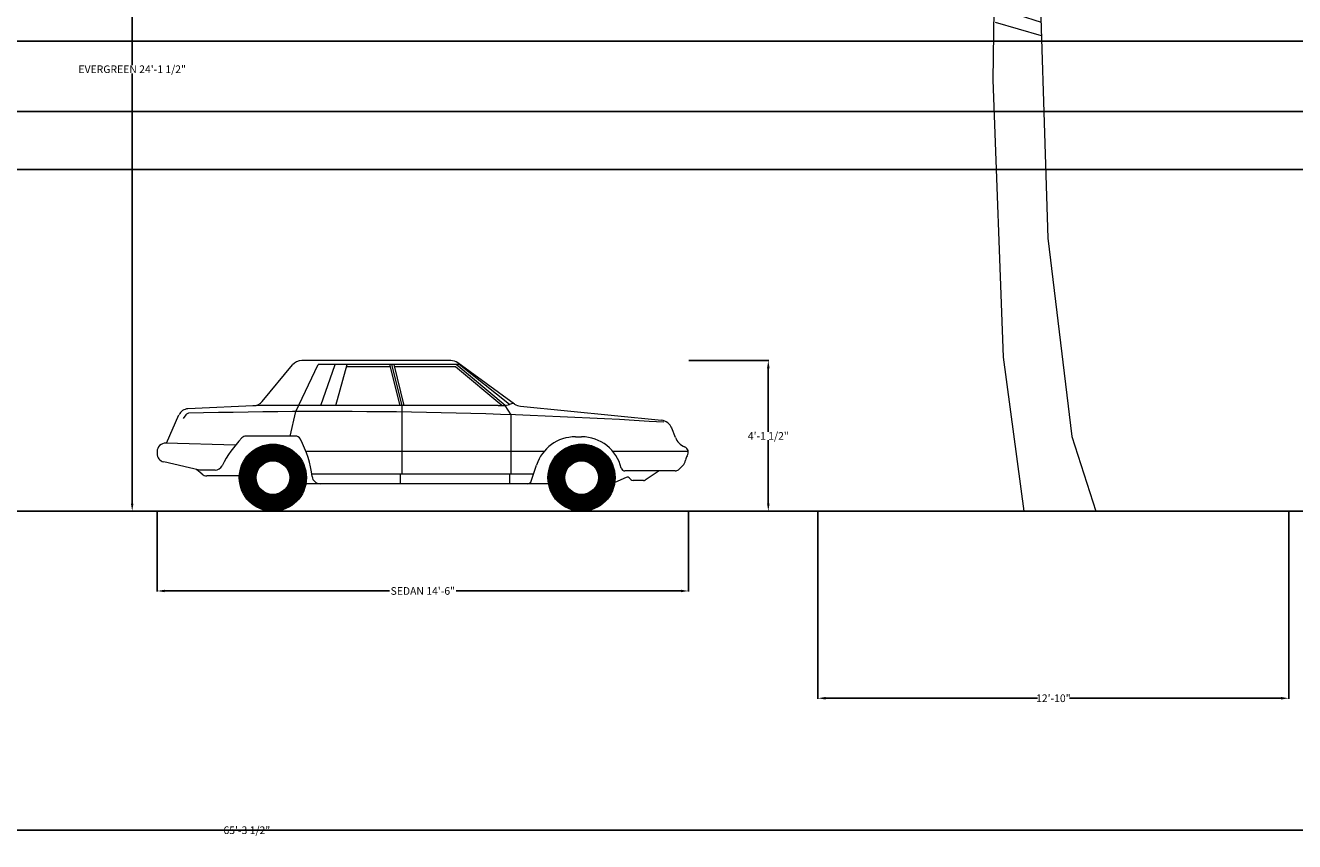
# Model space of a CAD drawing. Units: inches. Extents: x 481 to 2783, y 1975 to 3327.
# Tile 2 of 13: x 910 to 1326, y 2015 to 2282. Entities that reach past the tile are written whole.
import ezdxf

# ---------------------------------------------------------------- set-up
doc = ezdxf.new("R2010")
doc.units = ezdxf.units.IN
doc.header["$MEASUREMENT"] = 0
for name, color, linetype, lineweight in [('A-ANNO-DIMS', 50, 'Continuous', 18), ('A-ENTG', 7, 'Continuous', 13), ('C-TOPO', 7, 'Continuous', 25), ('L-PLNT', 7, 'Continuous', 13)]:
    doc.layers.add(name, color=color, linetype=linetype, lineweight=lineweight)
doc.styles.get("Standard").update_dxf_attribs({"font": 'arial.ttf'})
doc.dimstyles.get("Standard").update_dxf_attribs({"dimtxt": 2.5, "dimasz": 2.5, "dimexe": 0.18, "dimexo": 0.0625, "dimgap": 0.09, "dimtad": 0, "dimtih": 1, "dimtoh": 1, "dimzin": 0, "dimdsep": 46, "dimlunit": 3, "dimtxsty": 'Standard', "dimcen": 0.09, "dimadec": 0, "dimazin": 0, "dimtfac": 1, "dimtofl": 0, "dimtmove": 0, "dimatfit": 3, "dimfxl": 1, "dimtolj": 1, "dimtzin": 0, "dimarcsym": 0})

# ---------------------------------------------------------------- blocks, each defined once
blk = doc.blocks.new('Car - sedan  side')
for p, q in [((-139.53, 35.99), (-129.64, 47.91)), ((-128.57, 32.64), (-121.22, 48.02)), ((-77.81, 49.34), (-126.58, 49.34)), ((-74.7, 48.02), (-121.22, 48.02)), ((-120.32, 34.67), (-115.67, 48.02)), ((-115.4, 34.67), (-111.74, 48.02)), ((-97.55, 47.3), (-111.94, 47.3)), ((-94.41, 34.67), (-97.73, 48.02)), ((-93.72, 34.67), (-97.04, 48.02)), ((-93.03, 34.67), (-96.34, 48.02)), ((-76.26, 47.3), (-96.16, 47.3)), ((-61.08, 34.66), (-76.26, 47.3)), ((-60.02, 34.65), (-76.07, 48.02)), ((-56.87, 35.13), (-75.48, 48.59)), ((-58.54, 34.93), (-74.99, 48.02)), ((-140.23, 34.67), (-163.88, 33.56)), ((-62.28, 34.67), (-140.23, 34.67)), ((-93.72, 19.62), (-93.72, 34.67)), ((-62.28, 34.67), (-60.02, 34.65)), ((-60.02, 34.65), (-58.54, 34.93)), ((-57.97, 31.61), (-60.02, 34.65)), ((-57.21, 35.38), (-58.54, 34.93)), ((-54.93, 34.4), (-8.75, 29.8)), ((-170.93, 22.32), (-166.81, 31.56)), ((-164.57, 31.6), (-165.48, 30.35)), ((-130.39, 24.63), (-128.57, 32.64)), ((-57.97, 19.62), (-57.97, 31.61)), ((-4.21, 24.18), (-5.42, 27.27)), ((-148.26, 21.7), (-171.11, 22.33)), ((-128.78, 24.63), (-144.79, 24.63)), ((-36.97, 24.38), (-34.94, 24.38)), ((-174, 19.51), (-174, 18.91)), ((-47.2, 19.62), (-125.23, 19.62)), ((-93.72, 12.14), (-93.72, 19.62)), ((-57.97, 12.14), (-57.97, 19.62)), ((0, 19.62), (-24.7, 19.62)), ((-160.12, 13.48), (-171.81, 16.16)), ((-159.22, 12.14), (-161.08, 13.7)), ((-155.01, 13.48), (-160.12, 13.48)), ((-51.4, 9.89), (-49.69, 15.14)), ((-4.23, 13.19), (-20.72, 13.19)), ((-9.5, 13.19), (-14.1, 10.2)), ((-3.22, 13.59), (-1.77, 14.97)), ((-147.03, 11.6), (-157.73, 11.6)), ((-120.62, 9.03), (-125.23, 9.03)), ((-50.67, 12.14), (-123.32, 12.14)), ((-45.76, 9.03), (-120.62, 9.03)), ((-94.21, 9.03), (-94.21, 12.14)), ((-58.39, 9.03), (-58.39, 12.14)), ((-20.36, 11.06), (-24.06, 9.44)), ((-18.83, 10.42), (-19.11, 10.76)), ((-14.68, 10.03), (-18.01, 10.03))]:
    blk.add_line(p, q)
at = {"const_width": 5.49}
for points in [[(-127.8, 11, -1), (-144.3, 11, -1)], [(-26.69, 11, -1), (-43.19, 11, -1)]]:
    blk.add_lwpolyline(points, format="xyb", close=True, dxfattribs=at)
for centre, radius in [((-136.05, 11), 11), ((-34.94, 11), 11), ((-136.05, 11), 5.51), ((-34.94, 11), 5.51)]:
    blk.add_circle(centre, radius)
for centre, radius, start, end in [((-126.58, 45.38), 3.97, 90, 140.3029), ((-77.81, 45.38), 3.97, 54.135, 90), ((-163.72, 30.18), 3.38, 92.6827, 155.9736), ((-142.58, 38.53), 3.97, 272.6827, 320.3029), ((-54.54, 38.35), 3.97, 234.135, 264.3123), ((-163.62, 30.91), 1.17, 91.491, 143.9553), ((-118.51, -1702.12), 1734.79, 86.34698, 91.49105), ((-9.15, 25.82), 4, 21.3107, 84.3123), ((-171.18, 19.51), 2.82, 88.4193, 180), ((-118.09, -2.78), 38.85, 136.3964, 152.9097), ((-144.79, 22.64), 1.98, 90, 136.3964), ((-128.78, 22.64), 1.98, 28.1371, 90), ((-157.14, 7.48), 34.14, 6.5135, 28.1371), ((-36.97, 11), 13.38, 90, 161.9732), ((-34.94, 11), 13.38, 13.5864, 90), ((0.9, 26.18), 5.49, 201.3107, 247.7048), ((-1.92, 19.3), 1.94, 325.3744, 67.7048), ((-171.18, 18.91), 2.82, 180, 257.0905), ((-3.82, 17.12), 2.96, 313.7173, 352.3839), ((2.46, 16.28), 3.37, 145.3744, 172.3839), ((-155.01, 16.1), 2.62, 270, 332.9097), ((-20.72, 14.43), 1.24, 193.5864, 270), ((-4.23, 14.65), 1.46, 270, 313.7173), ((-157.73, 13.93), 2.32, 230.1291, 270), ((-120.62, 11.65), 2.62, 186.5135, 270), ((-52.58, 10.27), 1.24, 270, 341.9732), ((-19.93, 10.09), 1.06, 39.301, 113.7159), ((-18.01, 11.09), 1.06, 219.301, 270), ((-14.68, 11.09), 1.06, 270, 303.047)]:
    blk.add_arc(centre, radius, start, end)
blk = doc.blocks.new('Tree - palm elevation')
for p, q in [((-5.567, 196.707), (-4.987, 201.167)), ((-7.5, 199.68), (-7.5, 197.946)), ((-4.407, 195.716), (-3.247, 200.672)), ((-2.474, 193.733), (-1.315, 199.433)), ((15.116, 194.477), (17.822, 198.689)), ((18.015, 195.716), (20.914, 198.689)), ((-6.727, 197.202), (-11.366, 197.45)), ((-1.121, 190.759), (0.232, 196.955)), ((9.317, 191.255), (10.283, 196.955)), ((11.829, 192.99), (13.182, 197.45)), ((13.956, 194.229), (14.729, 196.955)), ((21.301, 196.459), (22.847, 198.441)), ((22.074, 196.707), (23.427, 195.716)), ((23.234, 196.707), (23.62, 197.698)), ((-3.441, 194.477), (-10.013, 195.716)), ((16.082, 194.972), (17.822, 192.494)), ((18.015, 195.468), (18.981, 192.494)), ((19.368, 196.459), (19.948, 193.733)), ((20.914, 196.459), (21.301, 194.972)), ((-20.064, 191.751), (-25.863, 193.238)), ((-15.232, 191.255), (-20.644, 193.981)), ((-9.433, 189.025), (-15.618, 193.238)), ((-1.894, 192.494), (-9.24, 193.733)), ((0.038, 188.281), (1.778, 193.981)), ((5.837, 187.786), (7.577, 194.229)), ((14.536, 193.981), (17.242, 191.255)), ((-29.729, 190.759), (-31.469, 191.255)), ((-30.309, 190.512), (-30.695, 189.025)), ((-25.283, 191.751), (-29.342, 192.246)), ((-28.763, 190.759), (-28.763, 188.281)), ((-26.443, 191.503), (-26.636, 186.051)), ((-23.737, 191.751), (-24.51, 185.06)), ((-21.031, 191.998), (-21.804, 183.325)), ((-17.551, 191.503), (-20.451, 181.343)), ((-14.265, 190.759), (-18.131, 182.086)), ((-0.541, 189.52), (-7.307, 192.494)), ((1.005, 185.803), (2.358, 190.759)), ((4.098, 185.06), (4.678, 190.512)), ((8.544, 190.512), (13.763, 189.52)), ((11.25, 192.494), (15.889, 190.512)), ((-11.753, 189.768), (-15.425, 182.83)), ((-6.147, 186.299), (-9.24, 190.264)), ((-5.76, 190.016), (0.618, 185.308)), ((6.997, 188.529), (12.216, 187.786)), ((15.695, 186.299), (19.368, 188.777)), ((19.368, 187.29), (26.133, 189.768)), ((24.78, 187.538), (31.546, 188.777)), ((-8.08, 188.034), (-12.912, 182.83)), ((-5.76, 188.034), (-1.508, 182.582)), ((1.005, 182.582), (2.938, 186.547)), ((4.871, 186.051), (10.09, 186.547)), ((9.51, 184.317), (15.502, 188.034)), ((17.242, 186.547), (23.041, 180.599)), ((20.721, 187.042), (25.167, 181.343)), ((23.814, 187.29), (26.907, 181.343)), ((26.133, 187.29), (29.419, 181.838)), ((28.066, 187.29), (30.966, 182.582)), ((29.806, 186.795), (32.319, 183.078)), ((29.999, 186.795), (33.092, 187.29)), ((-4.987, 185.803), (-10.979, 182.086)), ((-2.668, 185.803), (1.198, 181.343)), ((4.871, 181.591), (8.544, 184.812)), ((11.25, 184.812), (17.628, 180.352)), ((14.536, 185.803), (19.948, 180.847)), ((32.512, 186.299), (35.218, 186.299)), ((33.479, 186.051), (34.445, 182.83)), ((35.605, 185.556), (37.151, 185.308)), ((35.798, 185.308), (36.958, 181.591)), ((38.118, 184.317), (38.504, 181.838)), ((-3.247, 183.821), (-8.08, 181.838)), ((2.938, 182.582), (6.61, 183.821)), ((7.77, 183.325), (16.082, 179.856)), ((39.857, 182.83), (40.244, 181.591)), ((-1.315, 181.591), (-5.374, 181.095)), ((-0.348, 180.352), (-1.894, 180.104)), ((4.098, 180.847), (8.35, 179.608)), ((5.644, 181.838), (13.569, 178.865)), ((-15.618, 179.36), (-20.644, 178.617)), ((-17.358, 178.617), (-13.299, 173.661)), ((-15.038, 179.36), (-10.786, 174.404)), ((-12.332, 180.104), (-9.433, 175.643)), ((-10.206, 180.104), (-8.08, 175.891)), ((-8.273, 180.104), (-6.147, 176.635)), ((-6.34, 179.608), (-4.6, 177.13)), ((-4.021, 179.36), (-2.861, 177.378)), ((7.384, 178.369), (10.476, 179.36)), ((11.829, 177.874), (18.015, 179.113)), ((18.015, 177.13), (26.133, 179.113)), ((-21.031, 177.626), (-24.897, 176.387)), ((-22.191, 176.635), (-16.391, 169.448)), ((-20.064, 177.626), (-15.812, 172.67)), ((-1.701, 176.882), (-8.66, 175.396)), ((-2.668, 176.387), (-2.376, 170.594)), ((-0.928, 176.882), (-1.508, 173.909)), ((1.585, 177.13), (0.038, 174.652)), ((1.585, 177.13), (6.61, 176.139)), ((6.224, 178.121), (8.157, 175.148)), ((8.157, 178.121), (10.476, 172.422)), ((10.476, 177.874), (12.796, 169.696)), ((13.182, 177.874), (14.729, 166.97)), ((15.889, 177.13), (16.855, 164.492)), ((20.914, 175.891), (30.966, 176.635)), ((-25.09, 175.148), (-28.376, 174.404)), ((-25.476, 174.652), (-21.224, 167.466)), ((-24.317, 175.891), (-18.711, 168.457)), ((-4.214, 175.148), (-14.072, 170.935)), ((-4.6, 174.9), (-4.021, 166.722)), ((2.551, 175.891), (-0.928, 171.431)), ((3.711, 174.404), (-0.541, 167.961)), ((2.938, 175.891), (8.737, 173.413)), ((18.981, 175.891), (19.561, 163.005)), ((21.688, 175.396), (22.074, 161.518)), ((23.814, 174.404), (25.554, 160.279)), ((-28.956, 172.174), (-32.435, 170.192)), ((-27.409, 173.413), (-30.695, 172.67)), ((-27.989, 172.422), (-26.056, 166.227)), ((-26.829, 173.661), (-23.544, 167.218)), ((-6.92, 172.917), (-5.374, 163.253)), ((4.291, 173.909), (12.216, 168.953)), ((25.554, 173.661), (33.285, 173.661)), ((26.52, 173.165), (28.066, 159.784)), ((28.839, 172.174), (36.378, 170.687)), ((-29.922, 170.687), (-27.989, 165.235)), ((-8.466, 171.678), (-16.585, 167.713)), ((-8.853, 170.935), (-7.113, 160.527)), ((5.257, 171.926), (-0.155, 163.005)), ((6.417, 170.439), (14.729, 164.492)), ((29.226, 171.926), (30.966, 158.545)), ((30.966, 170.687), (38.891, 167.713)), ((-32.628, 167.961), (-33.208, 167.961)), ((-31.082, 169.944), (-32.435, 169.2)), ((-31.662, 168.705), (-31.082, 165.483)), ((-12.139, 167.961), (-19.098, 162.014)), ((-10.979, 168.457), (-7.887, 157.801)), ((7.384, 168.705), (0.812, 157.553)), ((32.126, 169.696), (32.512, 158.545)), ((34.058, 168.705), (34.445, 158.545)), ((-32.628, 167.713), (-32.435, 165.979)), ((-12.719, 166.722), (-9.046, 154.828)), ((8.544, 165.979), (16.662, 160.527)), ((35.412, 167.713), (41.404, 164.988)), ((36.378, 166.474), (35.605, 158.792)), ((-14.265, 164.244), (-19.678, 158.049)), ((9.317, 164.244), (2.358, 154.332)), ((37.731, 165.235), (36.958, 159.288)), ((37.924, 165.235), (41.404, 163.749)), ((38.504, 164.492), (38.504, 159.536)), ((-14.265, 163.749), (-10.786, 154.828)), ((10.09, 162.51), (17.435, 157.058)), ((39.664, 163.253), (42.37, 161.766)), ((39.857, 162.757), (39.857, 160.031)), ((-16.005, 160.031), (-19.484, 154.084)), ((-15.618, 160.775), (-12.332, 154.332)), ((10.863, 159.784), (4.484, 152.35)), ((40.824, 161.766), (41.21, 160.031)), ((41.21, 161.518), (42.757, 160.279)), ((-16.585, 158.545), (-13.106, 152.35)), ((-17.358, 155.819), (-14.845, 151.358)), ((11.443, 157.553), (16.855, 154.332)), ((11.829, 155.075), (6.804, 150.119)), ((-18.131, 153.589), (-19.484, 151.606)), ((-17.938, 152.597), (-16.972, 151.111)), ((12.216, 153.093), (16.082, 151.606)), ((12.603, 151.111), (8.544, 148.385)), ((12.603, 149.872), (15.116, 149.128)), ((12.216, 148.137), (10.09, 147.393)), ((12.409, 145.659), (11.056, 145.659)), ((12.409, 146.898), (13.763, 146.402)), ((-4.081, 140.645), (0.753, 138.261)), ((-4.081, 137.547), (0.753, 135.163)), ((-4.081, 129.205), (1.124, 126.821)), ((-4.081, 127.298), (1.31, 123.246)), ((-4.081, 121.578), (1.31, 120.863)), ((-4.267, 114.428), (1.682, 108.708)), ((-4.453, 112.283), (1.682, 105.133)), ((-4.639, 102.273), (1.868, 100.604)), ((-4.453, 99.651), (2.24, 98.459)), ((-4.453, 91.071), (2.426, 89.641)), ((-4.825, 83.921), (2.612, 81.061)), ((-4.639, 81.299), (2.797, 78.916)), ((-4.639, 78.916), (2.797, 76.771))]:
    blk.add_line(p, q)
for points in [[(-2.363, 170.553), (-3.88, 148.505), (-4.988, 69.634), (-3.325, 24.869), (0, 0)], [(-0.116, 162.848), (0.554, 143.532), (2.217, 96.635), (3.88, 44.054), (7.76, 12.079), (11.64, 0)]]:
    blk.add_lwpolyline(points)
for centre, radius, start, end in [((-18.427, 181.448), 19.715, 350.285, 64.11229), ((25.595, 171.567), 25.395, 91.40319, 163.882), ((-21.738, 166.094), 25.899, 27.67115, 112.5305), ((23.687, 155.341), 32.188, 56.19272, 134.3213), ((-9.259, 151.732), 28.386, 68.38311, 147.5322), ((14.394, 148.393), 32.752, 113.7592, 177.4133), ((5.828, 132.718), 45.639, 35.98777, 95.82273), ((-32.8, 147.923), 45.309, 356.1943, 41.37848)]:
    blk.add_arc(centre, radius, start, end)
blk = doc.blocks.new('*D54')
at = {"layer": 'A-ANNO-DIMS', "color": 0, "lineweight": -2, "transparency": 16777216}
for p, q in [((1324.1, 2531.22), (1385.48, 2531.22)), ((1385.3, 2528.72), (1385.3, 2328.4)), ((1385.3, 2125.32), (1385.3, 2325.64)), ((1324.1, 2122.82), (1385.48, 2122.82))]:
    blk.add_line(p, q, dxfattribs=at)
at = {"layer": 'A-ANNO-DIMS', "color": 0, "transparency": 16777216}
for points in [[(1384.88, 2528.72), (1385.72, 2528.72), (1385.3, 2531.22)], [(1384.88, 2125.32), (1385.72, 2125.32), (1385.3, 2122.82)]]:
    blk.add_solid(points, dxfattribs=at)
at = {"layer": 'Defpoints', "color": 0, "transparency": 16777216}
for p in [(1324.04, 2531.22), (1385.3, 2531.22), (1324.04, 2122.82)]:
    blk.add_point(p, dxfattribs=at)
at = {"layer": 'A-ANNO-DIMS', "color": 0, "transparency": 16777216, "insert": (1385.3, 2327.02), "char_height": 2.5, "attachment_point": 5}
blk.add_mtext('\\A1;PALM 34\'-0 1/2"', dxfattribs=at)
blk = doc.blocks.new('*D55')
at = {"layer": 'A-ANNO-DIMS', "color": 0, "lineweight": -2, "transparency": 16777216}
for p, q in [((1169.82, 2122.76), (1169.82, 2061.38)), ((1324.04, 2122.76), (1324.04, 2061.38)), ((1172.32, 2061.56), (1241.69, 2061.56)), ((1321.54, 2061.56), (1252.17, 2061.56))]:
    blk.add_line(p, q, dxfattribs=at)
at = {"layer": 'A-ANNO-DIMS', "color": 0, "transparency": 16777216}
for points in [[(1172.32, 2061.98), (1172.32, 2061.14), (1169.82, 2061.56)], [(1321.54, 2061.98), (1321.54, 2061.14), (1324.04, 2061.56)]]:
    blk.add_solid(points, dxfattribs=at)
at = {"layer": 'Defpoints', "color": 0, "transparency": 16777216}
for p in [(1169.82, 2122.82), (1324.04, 2122.82), (1324.04, 2061.56)]:
    blk.add_point(p, dxfattribs=at)
at = {"layer": 'A-ANNO-DIMS', "color": 0, "transparency": 16777216, "insert": (1246.93, 2061.56), "char_height": 2.5, "attachment_point": 5}
blk.add_mtext('\\A1;12\'-10"', dxfattribs=at)
blk = doc.blocks.new('*D58')
at = {"layer": 'A-ANNO-DIMS', "color": 0, "lineweight": -2, "transparency": 16777216}
for p, q in [((901.81, 2412.41), (945.37, 2412.41)), ((945.19, 2409.91), (945.19, 2269)), ((945.19, 2125.32), (945.19, 2266.23)), ((901.81, 2122.82), (945.37, 2122.82))]:
    blk.add_line(p, q, dxfattribs=at)
at = {"layer": 'A-ANNO-DIMS', "color": 0, "transparency": 16777216}
for points in [[(944.77, 2409.91), (945.61, 2409.91), (945.19, 2412.41)], [(944.77, 2125.32), (945.61, 2125.32), (945.19, 2122.82)]]:
    blk.add_solid(points, dxfattribs=at)
at = {"layer": 'Defpoints', "color": 0, "transparency": 16777216}
for p in [(901.75, 2412.41), (945.19, 2412.41), (901.75, 2122.82)]:
    blk.add_point(p, dxfattribs=at)
at = {"layer": 'A-ANNO-DIMS', "color": 0, "transparency": 16777216, "insert": (945.19, 2267.62), "char_height": 2.5, "attachment_point": 5}
blk.add_mtext('\\A1;EVERGREEN 24\'-1 1/2"', dxfattribs=at)
blk = doc.blocks.new('*D64')
at = {"layer": 'A-ANNO-DIMS', "color": 0, "lineweight": -2, "transparency": 16777216}
for p, q in [((953.33, 2122.76), (953.33, 2096.52)), ((1127.44, 2122.76), (1127.44, 2096.52)), ((955.83, 2096.7), (1029.51, 2096.7)), ((1124.94, 2096.7), (1051.27, 2096.7))]:
    blk.add_line(p, q, dxfattribs=at)
at = {"layer": 'A-ANNO-DIMS', "color": 0, "transparency": 16777216}
for points in [[(955.83, 2097.12), (955.83, 2096.29), (953.33, 2096.7)], [(1124.94, 2097.12), (1124.94, 2096.29), (1127.44, 2096.7)]]:
    blk.add_solid(points, dxfattribs=at)
at = {"layer": 'Defpoints', "color": 0, "transparency": 16777216}
for p in [(953.33, 2122.82), (1127.44, 2122.82), (1127.44, 2096.7)]:
    blk.add_point(p, dxfattribs=at)
at = {"layer": 'A-ANNO-DIMS', "color": 0, "transparency": 16777216, "insert": (1040.39, 2096.7), "char_height": 2.5, "attachment_point": 5}
blk.add_mtext('\\A1;SEDAN 14\'-6"', dxfattribs=at)
blk = doc.blocks.new('*D65')
at = {"layer": 'A-ANNO-DIMS', "color": 0, "lineweight": -2, "transparency": 16777216}
for p, q in [((1127.51, 2172.17), (1153.74, 2172.17)), ((1153.56, 2169.67), (1153.56, 2148.88)), ((1153.56, 2125.32), (1153.56, 2146.11)), ((1127.51, 2122.82), (1153.74, 2122.82))]:
    blk.add_line(p, q, dxfattribs=at)
at = {"layer": 'A-ANNO-DIMS', "color": 0, "transparency": 16777216}
for points in [[(1153.14, 2169.67), (1153.98, 2169.67), (1153.56, 2172.17)], [(1153.14, 2125.32), (1153.98, 2125.32), (1153.56, 2122.82)]]:
    blk.add_solid(points, dxfattribs=at)
at = {"layer": 'Defpoints', "color": 0, "transparency": 16777216}
for p in [(1127.44, 2172.17), (1153.56, 2172.17), (1127.44, 2122.82)]:
    blk.add_point(p, dxfattribs=at)
at = {"layer": 'A-ANNO-DIMS', "color": 0, "transparency": 16777216, "insert": (1153.56, 2147.49), "char_height": 2.5, "attachment_point": 5}
blk.add_mtext('\\A1;4\'-1 1/2"', dxfattribs=at)
blk = doc.blocks.new('*D66')
at = {"layer": 'A-ANNO-DIMS', "color": 0, "lineweight": -2, "transparency": 16777216}
for p, q in [((591.06, 2122.76), (591.06, 2018.14)), ((2669.26, 2122.76), (2669.26, 2018.14)), ((593.56, 2018.32), (1624.92, 2018.32)), ((2666.76, 2018.32), (1635.4, 2018.32))]:
    blk.add_line(p, q, dxfattribs=at)
at = {"layer": 'A-ANNO-DIMS', "color": 0, "transparency": 16777216}
for points in [[(593.56, 2018.74), (593.56, 2017.9), (591.06, 2018.32)], [(2666.76, 2018.74), (2666.76, 2017.9), (2669.26, 2018.32)]]:
    blk.add_solid(points, dxfattribs=at)
at = {"layer": 'Defpoints', "color": 0, "transparency": 16777216}
for p in [(591.06, 2122.82), (2669.26, 2122.82), (2669.26, 2018.32)]:
    blk.add_point(p, dxfattribs=at)
at = {"layer": 'A-ANNO-DIMS', "color": 0, "transparency": 16777216, "insert": (1630.16, 2018.32), "char_height": 2.5, "attachment_point": 5}
blk.add_mtext('\\A1;173\'-2"', dxfattribs=at)
blk = doc.blocks.new('*D67')
at = {"layer": 'A-ANNO-DIMS', "color": 0, "lineweight": -2, "transparency": 16777216}
for p, q in [((591.06, 2122.76), (591.06, 2018.14)), ((1374.44, 2122.76), (1374.44, 2018.14)), ((593.56, 2018.32), (975.45, 2018.32)), ((1371.94, 2018.32), (990.05, 2018.32))]:
    blk.add_line(p, q, dxfattribs=at)
at = {"layer": 'A-ANNO-DIMS', "color": 0, "transparency": 16777216}
for points in [[(593.56, 2018.74), (593.56, 2017.9), (591.06, 2018.32)], [(1371.94, 2018.74), (1371.94, 2017.9), (1374.44, 2018.32)]]:
    blk.add_solid(points, dxfattribs=at)
at = {"layer": 'Defpoints', "color": 0, "transparency": 16777216}
for p in [(591.06, 2122.82), (1374.44, 2122.82), (1374.44, 2018.32)]:
    blk.add_point(p, dxfattribs=at)
at = {"layer": 'A-ANNO-DIMS', "color": 0, "transparency": 16777216, "insert": (982.75, 2018.32), "char_height": 2.5, "attachment_point": 5}
blk.add_mtext('\\A1;65\'-3 1/2"', dxfattribs=at)
blk = doc.blocks.new('*D69')
at = {"layer": 'A-ANNO-DIMS', "color": 0, "lineweight": -2, "transparency": 16777216}
for p, q in [((1374.38, 2276.82), (486.38, 2276.82)), ((486.56, 2274.32), (486.56, 2201.19)), ((486.56, 2125.32), (486.56, 2198.45)), ((1374.38, 2122.82), (486.38, 2122.82))]:
    blk.add_line(p, q, dxfattribs=at)
at = {"layer": 'A-ANNO-DIMS', "color": 0, "transparency": 16777216}
for points in [[(486.15, 2274.32), (486.98, 2274.32), (486.56, 2276.82)], [(486.15, 2125.32), (486.98, 2125.32), (486.56, 2122.82)]]:
    blk.add_solid(points, dxfattribs=at)
at = {"layer": 'Defpoints', "color": 0, "transparency": 16777216}
for p in [(486.56, 2276.82), (1374.44, 2276.82), (1374.44, 2122.82)]:
    blk.add_point(p, dxfattribs=at)
at = {"layer": 'A-ANNO-DIMS', "color": 0, "transparency": 16777216, "insert": (486.56, 2199.82), "char_height": 2.5, "attachment_point": 5}
blk.add_mtext('\\A1;12\'-10"', dxfattribs=at)
blk = doc.blocks.new('*D73')
at = {"layer": 'A-ANNO-DIMS', "color": 0, "lineweight": -2, "transparency": 16777216}
for p, q in [((1392.88, 2253.82), (486.38, 2253.82)), ((486.56, 2251.32), (486.56, 2245.67)), ((486.56, 2237.32), (486.56, 2242.98)), ((1392.88, 2234.82), (486.38, 2234.82))]:
    blk.add_line(p, q, dxfattribs=at)
at = {"layer": 'A-ANNO-DIMS', "color": 0, "transparency": 16777216}
for points in [[(486.15, 2251.32), (486.98, 2251.32), (486.56, 2253.82)], [(486.15, 2237.32), (486.98, 2237.32), (486.56, 2234.82)]]:
    blk.add_solid(points, dxfattribs=at)
at = {"layer": 'Defpoints', "color": 0, "transparency": 16777216}
for p in [(486.56, 2253.82), (1392.94, 2253.82), (1392.94, 2234.82)]:
    blk.add_point(p, dxfattribs=at)
at = {"layer": 'A-ANNO-DIMS', "color": 0, "transparency": 16777216, "insert": (486.56, 2244.32), "char_height": 2.5, "attachment_point": 5}
blk.add_mtext('\\A1;1\'-7"', dxfattribs=at)

msp = doc.modelspace()

# ---------------------------------------------------------------- linework, layer by layer
at = {"layer": 'C-TOPO'}
msp.add_line((1374.438, 2122.821), (591.063, 2122.821), dxfattribs=at)
at = {"layer": 'L-PLNT'}
msp.add_line((1237.239, 2122.821), (1260.87, 2122.821), dxfattribs=at)

# ---------------------------------------------------------------- block references
at = {"layer": 'A-ENTG'}
msp.add_blockref('Car - sedan  side', (1127.33, 2122.821), dxfattribs=at)
at = {"layer": 'L-PLNT', "xscale": 2.030135039985482, "yscale": 2.030135039985482, "zscale": 2.030135039985482}
msp.add_blockref('Tree - palm elevation', (1237.239, 2122.821), dxfattribs=at)

# ---------------------------------------------------------------- dimensions: what is measured, and where the dimension line sits
at = {"layer": 'A-ANNO-DIMS'}
for base, p1, p2, text, picture, middle in [((1385.301, 2531.217), (1324.042, 2122.821), (1324.042, 2531.217), 'PALM <>', '*D54', (1385.301, 2327.019)), ((945.19, 2412.413), (901.751, 2122.821), (901.751, 2412.413), 'EVERGREEN <>', '*D58', (945.19, 2267.617))]:
    dim = msp.add_linear_dim(base=base, p1=p1, p2=p2, angle=90, text=text, dimstyle='Standard', override={"dimdec": 1, "dimlfac": 1, "dimrnd": 0, "dimzin": 1, "dimdsep": 46, "dimlunit": 4, "dimfrac": 2}, dxfattribs=at)
    dim.commit()
    dim.dimension.update_dxf_attribs({"geometry": picture, "text_midpoint": middle})
for base, p1, p2, picture, middle in [((486.563, 2276.821), (1374.438, 2122.821), (1374.438, 2276.821), '*D69', (486.563, 2199.821)), ((486.563, 2253.821), (1392.938, 2234.821), (1392.938, 2253.821), '*D73', (486.563, 2244.321)), ((1153.561, 2172.165), (1127.444, 2122.821), (1127.444, 2172.165), '*D65', (1153.561, 2147.493))]:
    dim = msp.add_linear_dim(base=base, p1=p1, p2=p2, angle=90, dimstyle='Standard', override={"dimdec": 1, "dimlfac": 1, "dimrnd": 0, "dimzin": 1, "dimdsep": 46, "dimlunit": 4, "dimfrac": 2}, dxfattribs=at)
    dim.commit()
    dim.dimension.update_dxf_attribs({"geometry": picture, "text_midpoint": middle})
for base, p1, p2, picture, middle in [((2669.257, 2018.321), (591.063, 2122.821), (2669.257, 2122.821), '*D66', (1630.16, 2018.321)), ((1374.438, 2018.321), (591.063, 2122.821), (1374.438, 2122.821), '*D67', (982.75, 2018.321)), ((1324.042, 2061.561), (1169.822, 2122.821), (1324.042, 2122.821), '*D55', (1246.932, 2061.561))]:
    dim = msp.add_linear_dim(base=base, p1=p1, p2=p2, dimstyle='Standard', override={"dimdec": 1, "dimlfac": 1, "dimrnd": 0, "dimzin": 1, "dimdsep": 46, "dimlunit": 4, "dimfrac": 2}, dxfattribs=at)
    dim.commit()
    dim.dimension.update_dxf_attribs({"geometry": picture, "text_midpoint": middle})
dim = msp.add_linear_dim(base=(1127.444, 2096.704), p1=(953.33, 2122.821), p2=(1127.444, 2122.821), text='SEDAN <>', dimstyle='Standard', override={"dimdec": 1, "dimlfac": 1, "dimrnd": 0, "dimzin": 1, "dimdsep": 46, "dimlunit": 4, "dimfrac": 2}, dxfattribs=at)
dim.commit()
dim.dimension.update_dxf_attribs({"geometry": '*D64', "text_midpoint": (1040.387, 2096.704)})

doc.saveas('drawing.dxf')
